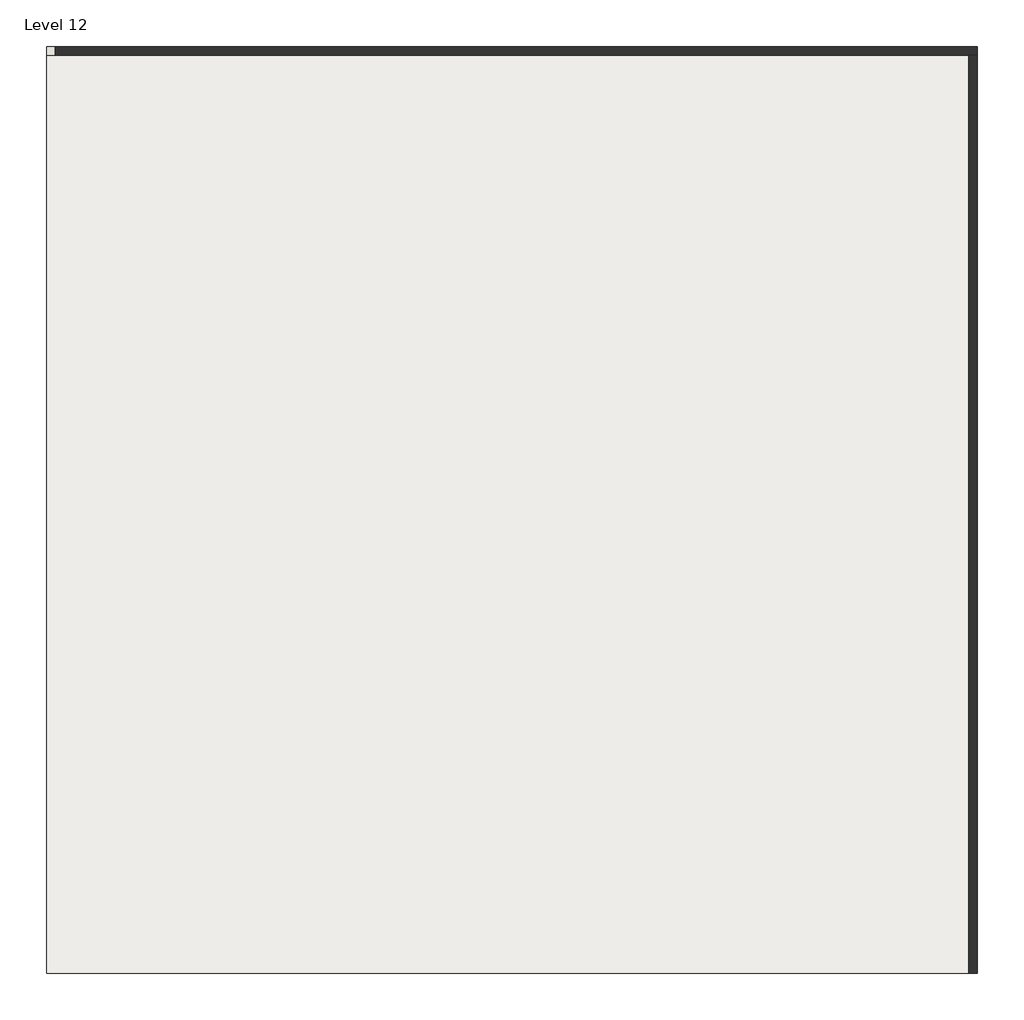
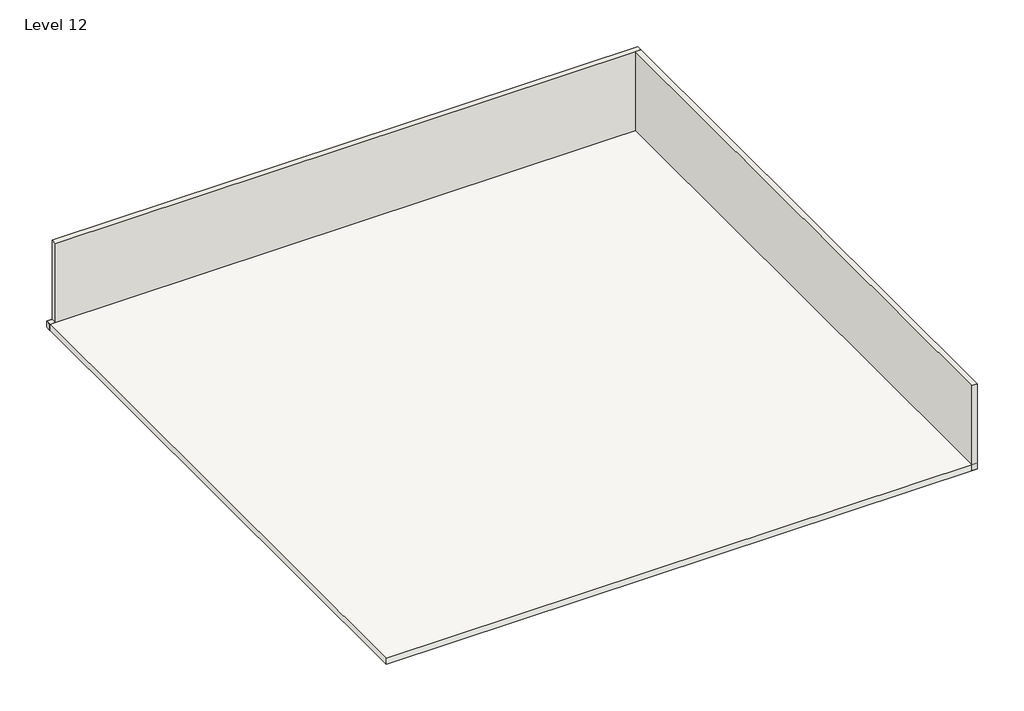
# One storey: 2 walls, 1 roof.
"""IFC4 building model written with IfcOpenShell, lengths in millimetres."""

from ifc_helpers import new_model, si_unit, frame, origin, place, context, project, spatial, polyline, outline, extrude, faceted_brep, element, save

model = new_model("IFC4")

# Units and contexts
model_context = context("Model", 3, world=origin())
ifc_project = project(units=[si_unit("LENGTHUNIT", "METRE", prefix="MILLI")], contexts=[model_context])

# Site, building, storey
site = spatial("IfcSite", under=ifc_project)
building = spatial("IfcBuilding", under=site)
storey = spatial("IfcBuildingStorey", under=building, Name="Level 12", Elevation=19431.0)

# Roof
placement = place(None, origin())
element("IfcRoof", 1, ObjectType="Generic - 9\"", at=placement, inside=storey, context=model_context, shape_type="SweptSolid", body=[
    extrude(outline(polyline([(-8934.7629849, 17755.0995758), (12604.4370151, 17755.0995758), (12604.4370151, -3682.5004242), (-8934.7629849, -3682.5004242), (-8934.7629849, 17755.0995758)])), frame((0.0, 0.0, 19431.0), z_axis=(0.0, 0.0, 1.0), x_axis=(1.0, 0.0, 0.0)), (0.0, 0.0, 1.0), 228.6),
])

# Walls
element("IfcWall", 2, ObjectType="outer wall", at=placement, inside=storey, context=model_context, shape_type="Brep", body=[
    faceted_brep([(-8934.7629849, 17551.8995758, 19431.0), (-8731.5629849, 17551.8995758, 19431.0), (12401.2370151, 17551.8995758, 19431.0), (12604.4370151, 17551.8995758, 19431.0), (12604.4370151, 17551.8995758, 22707.6), (12401.2370151, 17551.8995758, 22707.6), (-8731.5629849, 17551.8995758, 22707.6), (-8731.5629849, 17551.8995758, 19659.6), (-8934.7629849, 17551.8995758, 19659.6), (-8934.7629849, 17755.0995758, 19431.0), (-8934.7629849, 17755.0995758, 19659.6), (-8731.5629849, 17755.0995758, 19659.6), (-8731.5629849, 17755.0995758, 22707.6), (12604.4370151, 17755.0995758, 22707.6), (12604.4370151, 17755.0995758, 19431.0), (12401.2370151, 17755.0995758, 19431.0), (-8731.5629849, 17755.0995758, 19431.0)], [[[0, 1, 2, 3, 4, 5, 6, 7, 8]], [[9, 10, 11, 12, 13, 14, 15, 16]], [[3, 2, 1, 0, 9, 16, 15, 14]], [[6, 5, 4, 13, 12]], [[7, 11, 10, 8]], [[0, 8, 10, 9]], [[7, 6, 12, 11]], [[4, 3, 14, 13]]]),
])
element("IfcWall", 3, ObjectType="outer wall", at=placement, inside=storey, context=model_context, shape_type="SweptSolid", body=[
    extrude(outline(polyline([(12604.4370151, 17551.8995758), (12604.4370151, -3682.5004242), (12401.2370151, -3682.5004242), (12401.2370151, 17551.8995758), (12604.4370151, 17551.8995758)])), frame((0.0, 0.0, 19431.0), z_axis=(0.0, 0.0, 1.0), x_axis=(1.0, 0.0, 0.0)), (0.0, 0.0, 1.0), 3276.6),
])

save(model, "model.ifc")

# Revit data of these elements
# Type "Generic - 9\""
#   Assembly Code = "B1020"
#   Layers, outside or top first: 0' - 9" no material (function 1)
# Type "outer wall"
#   Assembly Code = "B2010"
#   Layers, outside or top first: 0' - 8" "Copper" (function 1)
# Element 1 (IfcRoof, "Generic - 9\"")
#   built-in parameter 1001705 = 64.5 (stored number, unit not read)
#   built-in parameter 1001710 = 33615
#   Phase Created = New Construction
#   Materials on its faces: "Default Roof"
# Elements 2, 3 (IfcWall, "outer wall")
#   Top Offset = 0' - 0"
#   Base Offset = 0' - 0"
#   Unconnected Height = 10' - 9"
#   wall height = 10' - 9"
#   Phase Created = New Construction
#   Base Constraint = Level 12
#   Materials on its faces: "Copper"
# Materials
#   "Copper": class "Metal", colour RGB 0 0 0, transparency 0, Description = "Copper, matte finish", Cost = 0
#   "Default Roof": colour RGB 88 101 114, transparency 0
